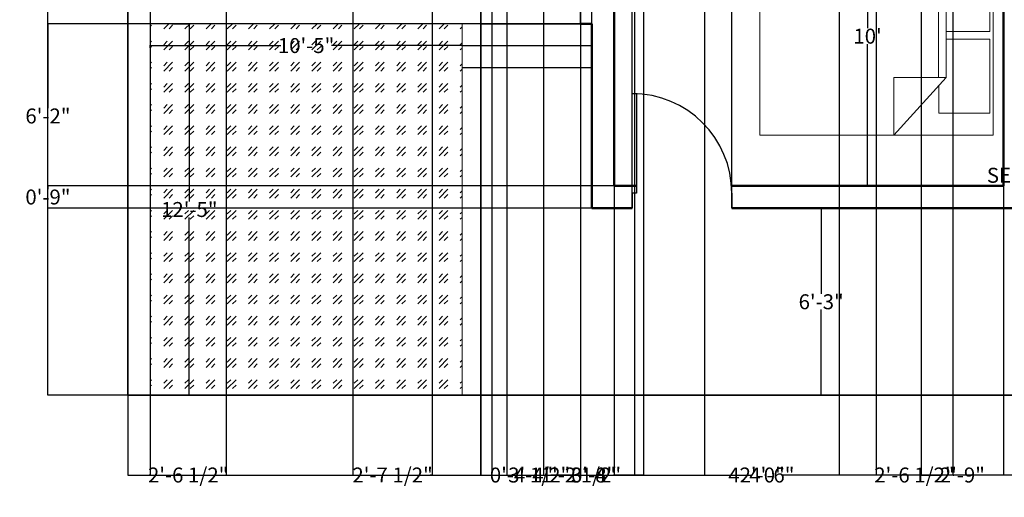
# Model space of a CAD drawing. Units: inches. Extents: x -56 to 545, y -536 to 185.
# Tile 1 of 7: x -49 to 345, y -536 to -344. Entities that reach past the tile are written whole.
import ezdxf

# ---------------------------------------------------------------- set-up
doc = ezdxf.new("R2010")
doc.units = ezdxf.units.IN
doc.header["$MEASUREMENT"] = 0
for name, color, linetype, lineweight in [('A-ANNO-DIMS', 2, 'Continuous', 18), ('A-DOOR', 4, 'Continuous', 25), ('A-FLOR-STRS', 7, 'Continuous', 25), ('A-FURN', 8, 'Continuous', 18), ('A-WALL', 7, 'Continuous', 50), ('C-PROP', 7, 'Continuous', 35), ('L-PLNT-PATT', 3, 'Continuous', 13), ('L-PLNT-TURF', 3, 'Continuous', 18)]:
    doc.layers.add(name, color=color, linetype=linetype, lineweight=lineweight)
doc.styles.get("Standard").update_dxf_attribs({"font": 'arial.ttf'})
doc.dimstyles.get("Standard").update_dxf_attribs({"dimtxt": 6, "dimasz": 0.18, "dimexe": 0.18, "dimexo": 0.0625, "dimgap": 0.09, "dimtad": 0, "dimtih": 1, "dimtoh": 1, "dimdec": 0, "dimzin": 0, "dimdsep": 46, "dimlunit": 3, "dimtxsty": 'Standard', "dimcen": 0.09, "dimclrd": 3, "dimclre": 3, "dimclrt": 3, "dimadec": 0, "dimazin": 0, "dimtfac": 1, "dimtdec": 0, "dimtofl": 0, "dimtmove": 0, "dimatfit": 3, "dimfxl": 1, "dimtolj": 1, "dimtzin": 0, "dimarcsym": 0})

# ---------------------------------------------------------------- blocks, each defined once
blk = doc.blocks.new('CAMAKING')
for points in [[(0.8635, 0), (-0.8635, 0)], [(-0.8635, -2.0147), (-0.8635, 0)], [(0.8635, 0), (0.8635, -2.0147)], [(-0.6723, -0.4077), (-0.6723, -0.0281)], [(-0.6723, -0.0281), (-0.0328, -0.0281)], [(-0.0328, -0.0281), (-0.0328, -0.4077)], [(0.6716, -0.027), (0.0319, -0.027)], [(0.0319, -0.027), (0.0319, -0.4077)], [(0.6716, -0.4686), (0.6716, -0.027)], [(0.3645, -0.4056), (-0.8635, -0.4056)], [(0.8635, -0.857), (0.3645, -0.4056)], [(0.3645, -0.4702), (0.3645, -0.4056)], [(-0.8635, -0.4702), (0.3645, -0.4702)], [(0.3645, -0.4702), (0.3645, -0.857)], [(0.4362, -0.4686), (0.6716, -0.4686)], [(0.3645, -0.857), (0.8635, -0.857)], [(0.8635, -2.0147), (-0.8635, -2.0147)]]:
    blk.add_lwpolyline(points)
blk = doc.blocks.new('*U7')
for p, q in [((0, 0), (0, -6)), ((40, 0), (40, -6))]:
    blk.add_line(p, q)
blk.add_lwpolyline([(0, 0), (0, 40), (1.75, 40), (1.75, 0)], close=True)
blk.add_arc((0, 0), 40, 0, 90)
blk = doc.blocks.new('*D14')
at = {"layer": 'A-ANNO-DIMS', "color": 0, "lineweight": -2, "transparency": 16777216}
for p, q in [((290.53, -291.02), (290.53, -347.69)), ((290.6, -290.84), (290.71, -290.84)), ((290.53, -410.66), (290.53, -353.99)), ((290.6, -410.84), (290.71, -410.84))]:
    blk.add_line(p, q, dxfattribs=at)
at = {"layer": 'A-ANNO-DIMS', "color": 0, "transparency": 16777216}
for points in [[(290.5, -291.02), (290.56, -291.02), (290.53, -290.84)], [(290.5, -410.66), (290.56, -410.66), (290.53, -410.84)]]:
    blk.add_solid(points, dxfattribs=at)
at = {"layer": 'Defpoints', "color": 0, "transparency": 16777216}
for p in [(290.53, -290.84), (290.53, -290.84), (290.53, -410.84)]:
    blk.add_point(p, dxfattribs=at)
at = {"layer": 'A-ANNO-DIMS', "color": 0, "transparency": 16777216, "insert": (290.53, -350.84), "char_height": 6, "attachment_point": 5}
blk.add_mtext("\\A1;10'", dxfattribs=at)
blk = doc.blocks.new('*D15')
at = {"layer": 'A-ANNO-DIMS', "color": 0, "lineweight": -2, "transparency": 16777216}
for p, q in [((11.7, -345.84), (18.9, -345.84)), ((18.72, -346.02), (18.72, -417.19)), ((18.72, -494.66), (18.72, -423.49)), ((11.7, -494.84), (18.9, -494.84))]:
    blk.add_line(p, q, dxfattribs=at)
at = {"layer": 'A-ANNO-DIMS', "color": 0, "transparency": 16777216}
for points in [[(18.69, -346.02), (18.75, -346.02), (18.72, -345.84)], [(18.69, -494.66), (18.75, -494.66), (18.72, -494.84)]]:
    blk.add_solid(points, dxfattribs=at)
at = {"layer": 'Defpoints', "color": 0, "transparency": 16777216}
for p in [(11.63, -345.84), (11.63, -494.84), (18.72, -494.84)]:
    blk.add_point(p, dxfattribs=at)
at = {"layer": 'A-ANNO-DIMS', "color": 0, "transparency": 16777216, "insert": (18.72, -420.34), "char_height": 6, "attachment_point": 5}
blk.add_mtext('\\A1;12\'-5"', dxfattribs=at)
blk = doc.blocks.new('*D16')
at = {"layer": 'A-ANNO-DIMS', "color": 0, "lineweight": -2, "transparency": 16777216}
for p, q in [((3.03, -355.56), (3.03, -354.43)), ((3.21, -354.61), (55.42, -354.61)), ((127.85, -354.61), (75.65, -354.61)), ((128.03, -354.55), (128.03, -354.43))]:
    blk.add_line(p, q, dxfattribs=at)
at = {"layer": 'A-ANNO-DIMS', "color": 0, "transparency": 16777216}
for points in [[(3.21, -354.58), (3.21, -354.64), (3.03, -354.61)], [(127.85, -354.58), (127.85, -354.64), (128.03, -354.61)]]:
    blk.add_solid(points, dxfattribs=at)
at = {"layer": 'Defpoints', "color": 0, "transparency": 16777216}
for p in [(128.03, -354.61), (128.03, -354.61), (3.03, -355.62)]:
    blk.add_point(p, dxfattribs=at)
at = {"layer": 'A-ANNO-DIMS', "color": 0, "transparency": 16777216, "insert": (65.53, -354.61), "char_height": 6, "attachment_point": 5}
blk.add_mtext('\\A1;10\'-5"', dxfattribs=at)
blk = doc.blocks.new('*D34')
at = {"layer": 'A-ANNO-DIMS', "color": 0, "lineweight": -2, "transparency": 16777216}
for p, q in [((263.14, -419.84), (272.12, -419.84)), ((271.94, -420.02), (271.94, -454.19)), ((271.94, -494.66), (271.94, -460.5)), ((263.14, -494.84), (272.12, -494.84))]:
    blk.add_line(p, q, dxfattribs=at)
at = {"layer": 'A-ANNO-DIMS', "color": 0, "transparency": 16777216}
for points in [[(271.91, -420.02), (271.97, -420.02), (271.94, -419.84)], [(271.91, -494.66), (271.97, -494.66), (271.94, -494.84)]]:
    blk.add_solid(points, dxfattribs=at)
at = {"layer": 'Defpoints', "color": 0, "transparency": 16777216}
for p in [(263.08, -419.84), (263.08, -494.84), (271.94, -494.84)]:
    blk.add_point(p, dxfattribs=at)
at = {"layer": 'A-ANNO-DIMS', "color": 0, "transparency": 16777216, "insert": (271.94, -457.34), "char_height": 6, "attachment_point": 5}
blk.add_mtext('\\A1;6\'-3"', dxfattribs=at)
blk = doc.blocks.new('*D49')
at = {"layer": 'A-ANNO-DIMS', "color": 3, "lineweight": -2, "transparency": 16777216}
for p, q in [((389.1, -321.67), (363.5, -321.67)), ((363.68, -321.85), (363.68, -403.43)), ((363.68, -491.39), (363.68, -409.81)), ((389.1, -491.57), (363.5, -491.57))]:
    blk.add_line(p, q, dxfattribs=at)
at = {"layer": 'A-ANNO-DIMS', "color": 3, "transparency": 16777216}
for points in [[(363.65, -321.85), (363.71, -321.85), (363.68, -321.67)], [(363.65, -491.39), (363.71, -491.39), (363.68, -491.57)]]:
    blk.add_solid(points, dxfattribs=at)
at = {"layer": 'Defpoints', "color": 0, "transparency": 16777216}
for p in [(389.16, -321.67), (363.68, -491.57), (389.16, -491.57)]:
    blk.add_point(p, dxfattribs=at)
at = {"layer": 'A-ANNO-DIMS', "color": 3, "transparency": 16777216, "insert": (363.68, -406.62), "char_height": 6, "attachment_point": 5}
blk.add_mtext('\\A1;SEDAN 14\'-2"', dxfattribs=at)
blk = doc.blocks.new('*D51')
at = {"layer": 'A-ANNO-DIMS', "color": 3, "lineweight": -2, "transparency": 16777216}
for p, q in [((498.03, -491.9), (498.03, -526.99)), ((-5.97, -494.9), (-5.97, -526.99)), ((-5.79, -526.81), (235.52, -526.81)), ((497.85, -526.81), (256.55, -526.81))]:
    blk.add_line(p, q, dxfattribs=at)
at = {"layer": 'A-ANNO-DIMS', "color": 3, "transparency": 16777216}
for points in [[(-5.79, -526.78), (-5.79, -526.84), (-5.97, -526.81)], [(497.85, -526.78), (497.85, -526.84), (498.03, -526.81)]]:
    blk.add_solid(points, dxfattribs=at)
at = {"layer": 'Defpoints', "color": 0, "transparency": 16777216}
for p in [(498.03, -491.84), (-5.97, -494.84), (498.03, -526.81)]:
    blk.add_point(p, dxfattribs=at)
at = {"layer": 'A-ANNO-DIMS', "color": 3, "transparency": 16777216, "insert": (246.03, -526.81), "char_height": 6, "attachment_point": 5}
blk.add_mtext('\\A1;42\'-0"', dxfattribs=at)
blk = doc.blocks.new('*D52')
at = {"layer": 'A-ANNO-DIMS', "color": 3, "lineweight": -2, "transparency": 16777216}
for p, q in [((-6.03, 93.16), (-38.11, 93.16)), ((-37.93, 92.98), (-37.93, -197.69)), ((-37.93, -494.66), (-37.93, -203.99)), ((-6.03, -494.84), (-38.11, -494.84))]:
    blk.add_line(p, q, dxfattribs=at)
at = {"layer": 'A-ANNO-DIMS', "color": 3, "transparency": 16777216}
for points in [[(-37.96, 92.98), (-37.9, 92.98), (-37.93, 93.16)], [(-37.96, -494.66), (-37.9, -494.66), (-37.93, -494.84)]]:
    blk.add_solid(points, dxfattribs=at)
at = {"layer": 'Defpoints', "color": 0, "transparency": 16777216}
for p in [(-5.97, 93.16), (-37.93, -494.84), (-5.97, -494.84)]:
    blk.add_point(p, dxfattribs=at)
at = {"layer": 'A-ANNO-DIMS', "color": 3, "transparency": 16777216, "insert": (-37.93, -200.84), "char_height": 6, "attachment_point": 5}
blk.add_mtext('\\A1;49\'-0"', dxfattribs=at)
blk = doc.blocks.new('*D53')
at = {"layer": 'A-ANNO-DIMS', "color": 3, "lineweight": -2, "transparency": 16777216}
for p, q in [((179.97, -345.84), (-38.11, -345.84)), ((-37.93, -346.02), (-37.93, -379.69)), ((-37.93, -419.66), (-37.93, -385.99)), ((179.97, -419.84), (-38.11, -419.84))]:
    blk.add_line(p, q, dxfattribs=at)
at = {"layer": 'A-ANNO-DIMS', "color": 3, "transparency": 16777216}
for points in [[(-37.96, -346.02), (-37.9, -346.02), (-37.93, -345.84)], [(-37.96, -419.66), (-37.9, -419.66), (-37.93, -419.84)]]:
    blk.add_solid(points, dxfattribs=at)
at = {"layer": 'Defpoints', "color": 0, "transparency": 16777216}
for p in [(180.03, -345.84), (-37.93, -419.84), (180.03, -419.84)]:
    blk.add_point(p, dxfattribs=at)
at = {"layer": 'A-ANNO-DIMS', "color": 3, "transparency": 16777216, "insert": (-37.93, -382.84), "char_height": 6, "attachment_point": 5}
blk.add_mtext('\\A1;6\'-2"', dxfattribs=at)
blk = doc.blocks.new('*D54')
at = {"layer": 'A-ANNO-DIMS', "color": 3, "lineweight": -2, "transparency": 16777216}
for p, q in [((188.97, -410.84), (-38.11, -410.84)), ((-37.93, -411.02), (-37.93, -412.19)), ((179.97, -419.84), (-38.11, -419.84)), ((-37.93, -419.66), (-37.93, -418.49))]:
    blk.add_line(p, q, dxfattribs=at)
at = {"layer": 'A-ANNO-DIMS', "color": 3, "transparency": 16777216}
for points in [[(-37.96, -411.02), (-37.9, -411.02), (-37.93, -410.84)], [(-37.96, -419.66), (-37.9, -419.66), (-37.93, -419.84)]]:
    blk.add_solid(points, dxfattribs=at)
at = {"layer": 'Defpoints', "color": 0, "transparency": 16777216}
for p in [(189.03, -410.84), (-37.93, -419.84), (180.03, -419.84)]:
    blk.add_point(p, dxfattribs=at)
at = {"layer": 'A-ANNO-DIMS', "color": 3, "transparency": 16777216, "insert": (-37.93, -415.34), "char_height": 6, "attachment_point": 5}
blk.add_mtext('\\A1;0\'-9"', dxfattribs=at)
blk = doc.blocks.new('*D60')
at = {"layer": 'A-ANNO-DIMS', "color": 3, "lineweight": -2, "transparency": 16777216}
for p, q in [((135.54, -345.9), (135.54, -526.99)), ((175.54, -345.9), (175.54, -526.99)), ((135.72, -526.81), (147.48, -526.81)), ((175.36, -526.81), (163.61, -526.81))]:
    blk.add_line(p, q, dxfattribs=at)
at = {"layer": 'A-ANNO-DIMS', "color": 3, "transparency": 16777216}
for points in [[(135.72, -526.78), (135.72, -526.84), (135.54, -526.81)], [(175.36, -526.78), (175.36, -526.84), (175.54, -526.81)]]:
    blk.add_solid(points, dxfattribs=at)
at = {"layer": 'Defpoints', "color": 0, "transparency": 16777216}
for p in [(135.54, -345.84), (175.54, -345.84), (175.54, -526.81)]:
    blk.add_point(p, dxfattribs=at)
at = {"layer": 'A-ANNO-DIMS', "color": 3, "transparency": 16777216, "insert": (155.54, -526.81), "char_height": 6, "attachment_point": 5}
blk.add_mtext('\\A1;3\'-4"', dxfattribs=at)
blk = doc.blocks.new('*D61')
at = {"layer": 'A-ANNO-DIMS', "color": 3, "lineweight": -2, "transparency": 16777216}
for p, q in [((175.54, -345.78), (175.54, 176.3)), ((175.72, 176.12), (179.85, 176.12)), ((180.03, -345.78), (180.03, 176.3)), ((180.03, 176.12), (180.21, 176.12))]:
    blk.add_line(p, q, dxfattribs=at)
at = {"layer": 'A-ANNO-DIMS', "color": 3, "transparency": 16777216}
for points in [[(175.72, 176.15), (175.72, 176.09), (175.54, 176.12)], [(179.85, 176.15), (179.85, 176.09), (180.03, 176.12)]]:
    blk.add_solid(points, dxfattribs=at)
at = {"layer": 'Defpoints', "color": 0, "transparency": 16777216}
for p in [(180.03, 176.12), (175.54, -345.84), (180.03, -345.84)]:
    blk.add_point(p, dxfattribs=at)
at = {"layer": 'A-ANNO-DIMS', "color": 3, "transparency": 16777216, "insert": (195.27, 176.12), "char_height": 6, "attachment_point": 5}
blk.add_mtext('\\A1;0\'-4 1/2"', dxfattribs=at)
blk = doc.blocks.new('*D62')
at = {"layer": 'A-ANNO-DIMS', "color": 3, "lineweight": -2, "transparency": 16777216}
for p, q in [((196.14, -419.78), (196.14, 176.3)), ((196.32, 176.12), (208.08, 176.12)), ((235.96, 176.12), (224.21, 176.12)), ((236.14, -419.78), (236.14, 176.3))]:
    blk.add_line(p, q, dxfattribs=at)
at = {"layer": 'A-ANNO-DIMS', "color": 3, "transparency": 16777216}
for points in [[(196.32, 176.15), (196.32, 176.09), (196.14, 176.12)], [(235.96, 176.15), (235.96, 176.09), (236.14, 176.12)]]:
    blk.add_solid(points, dxfattribs=at)
at = {"layer": 'Defpoints', "color": 0, "transparency": 16777216}
for p in [(236.14, 176.12), (196.14, -419.84), (236.14, -419.84)]:
    blk.add_point(p, dxfattribs=at)
at = {"layer": 'A-ANNO-DIMS', "color": 3, "transparency": 16777216, "insert": (216.14, 176.12), "char_height": 6, "attachment_point": 5}
blk.add_mtext('\\A1;3\'-4"', dxfattribs=at)
blk = doc.blocks.new('*D63')
at = {"layer": 'A-ANNO-DIMS', "color": 3, "lineweight": -2, "transparency": 16777216}
for p, q in [((189.03, -410.78), (189.03, 176.3)), ((189.21, 176.12), (195.96, 176.12)), ((196.14, -419.78), (196.14, 176.3)), ((196.14, 176.12), (196.32, 176.12))]:
    blk.add_line(p, q, dxfattribs=at)
at = {"layer": 'A-ANNO-DIMS', "color": 3, "transparency": 16777216}
for points in [[(189.21, 176.15), (189.21, 176.09), (189.03, 176.12)], [(195.96, 176.15), (195.96, 176.09), (196.14, 176.12)]]:
    blk.add_solid(points, dxfattribs=at)
at = {"layer": 'Defpoints', "color": 0, "transparency": 16777216}
for p in [(196.14, 176.12), (189.03, -410.84), (196.14, -419.84)]:
    blk.add_point(p, dxfattribs=at)
at = {"layer": 'A-ANNO-DIMS', "color": 3, "transparency": 16777216, "insert": (204.39, 176.12), "char_height": 6, "attachment_point": 5}
blk.add_mtext('\\A1;0\'-7"', dxfattribs=at)
blk = doc.blocks.new('*D64')
at = {"layer": 'A-ANNO-DIMS', "color": 3, "lineweight": -2, "transparency": 16777216}
for p, q in [((293.965457, -119.903074), (293.965457, -526.985574)), ((324.688571, -119.903074), (324.688571, -526.985574)), ((293.785457, -526.805574), (293.605457, -526.805574)), ((324.868571, -526.805574), (325.048571, -526.805574))]:
    blk.add_line(p, q, dxfattribs=at)
at = {"layer": 'A-ANNO-DIMS', "color": 3, "transparency": 16777216}
for points in [[(293.785457, -526.775574), (293.785457, -526.835574), (293.965457, -526.805574)], [(324.868571, -526.775574), (324.868571, -526.835574), (324.688571, -526.805574)]]:
    blk.add_solid(points, dxfattribs=at)
at = {"layer": 'Defpoints', "color": 0, "transparency": 16777216}
for p in [(293.965457, -119.840574), (324.688571, -119.840574), (324.688571, -526.805574)]:
    blk.add_point(p, dxfattribs=at)
at = {"layer": 'A-ANNO-DIMS', "color": 3, "transparency": 16777216, "insert": (309.327014, -526.805574), "char_height": 6, "attachment_point": 5}
blk.add_mtext('\\A1;2\'-6 1/2"', dxfattribs=at)
blk = doc.blocks.new('*D65')
at = {"layer": 'A-ANNO-DIMS', "color": 3, "lineweight": -2, "transparency": 16777216}
for p, q in [((160.69, -65.9), (160.69, -526.99)), ((200.69, -65.9), (200.69, -526.99)), ((160.87, -526.81), (172.63, -526.81)), ((200.51, -526.81), (188.76, -526.81))]:
    blk.add_line(p, q, dxfattribs=at)
at = {"layer": 'A-ANNO-DIMS', "color": 3, "transparency": 16777216}
for points in [[(160.87, -526.78), (160.87, -526.84), (160.69, -526.81)], [(200.51, -526.78), (200.51, -526.84), (200.69, -526.81)]]:
    blk.add_solid(points, dxfattribs=at)
at = {"layer": 'Defpoints', "color": 0, "transparency": 16777216}
for p in [(160.69, -65.84), (200.69, -65.84), (200.69, -526.81)]:
    blk.add_point(p, dxfattribs=at)
at = {"layer": 'A-ANNO-DIMS', "color": 3, "transparency": 16777216, "insert": (180.69, -526.81), "char_height": 6, "attachment_point": 5}
blk.add_mtext('\\A1;3\'-4"', dxfattribs=at)
blk = doc.blocks.new('*D66')
at = {"layer": 'A-ANNO-DIMS', "color": 3, "lineweight": -2, "transparency": 16777216}
for p, q in [((146.03, -65.9), (146.03, -526.99)), ((160.69, -65.9), (160.69, -526.99)), ((146.21, -526.81), (160.51, -526.81)), ((160.69, -526.81), (160.87, -526.81))]:
    blk.add_line(p, q, dxfattribs=at)
at = {"layer": 'A-ANNO-DIMS', "color": 3, "transparency": 16777216}
for points in [[(146.21, -526.78), (146.21, -526.84), (146.03, -526.81)], [(160.51, -526.78), (160.51, -526.84), (160.69, -526.81)]]:
    blk.add_solid(points, dxfattribs=at)
at = {"layer": 'Defpoints', "color": 0, "transparency": 16777216}
for p in [(146.03, -65.84), (160.69, -65.84), (160.69, -526.81)]:
    blk.add_point(p, dxfattribs=at)
at = {"layer": 'A-ANNO-DIMS', "color": 3, "transparency": 16777216, "insert": (175.65, -526.81), "char_height": 6, "attachment_point": 5}
blk.add_mtext('\\A1;1\'-2 1/2"', dxfattribs=at)
blk = doc.blocks.new('*D69')
at = {"layer": 'A-ANNO-DIMS', "color": 3, "lineweight": -2, "transparency": 16777216}
for p, q in [((189.03, -290.9), (189.03, -526.99)), ((197.13, -290.9), (197.13, -526.99)), ((189.03, -526.81), (188.85, -526.81)), ((196.95, -526.81), (189.21, -526.81))]:
    blk.add_line(p, q, dxfattribs=at)
at = {"layer": 'A-ANNO-DIMS', "color": 3, "transparency": 16777216}
for points in [[(189.21, -526.78), (189.21, -526.84), (189.03, -526.81)], [(196.95, -526.78), (196.95, -526.84), (197.13, -526.81)]]:
    blk.add_solid(points, dxfattribs=at)
at = {"layer": 'Defpoints', "color": 0, "transparency": 16777216}
for p in [(189.03, -290.84), (197.13, -290.84), (189.03, -526.81)]:
    blk.add_point(p, dxfattribs=at)
at = {"layer": 'A-ANNO-DIMS', "color": 3, "transparency": 16777216, "insert": (180.79, -526.81), "char_height": 6, "attachment_point": 5}
blk.add_mtext('\\A1;0\'-8"', dxfattribs=at)
blk = doc.blocks.new('*D73')
at = {"layer": 'A-ANNO-DIMS', "color": 3, "lineweight": -2, "transparency": 16777216}
for p, q in [((135.38, 28.1), (135.38, -526.99)), ((140.03, 28.1), (140.03, -526.99)), ((135.56, -526.81), (139.85, -526.81)), ((140.03, -526.81), (140.21, -526.81))]:
    blk.add_line(p, q, dxfattribs=at)
at = {"layer": 'A-ANNO-DIMS', "color": 3, "transparency": 16777216}
for points in [[(135.56, -526.78), (135.56, -526.84), (135.38, -526.81)], [(139.85, -526.78), (139.85, -526.84), (140.03, -526.81)]]:
    blk.add_solid(points, dxfattribs=at)
at = {"layer": 'Defpoints', "color": 0, "transparency": 16777216}
for p in [(135.38, 28.16), (140.03, 28.16), (140.03, -526.81)]:
    blk.add_point(p, dxfattribs=at)
at = {"layer": 'A-ANNO-DIMS', "color": 3, "transparency": 16777216, "insert": (155.27, -526.81), "char_height": 6, "attachment_point": 5}
blk.add_mtext('\\A1;0\'-4 1/2"', dxfattribs=at)
blk = doc.blocks.new('*D75')
at = {"layer": 'A-ANNO-DIMS', "color": 3, "lineweight": -2, "transparency": 16777216}
for p, q in [((33.5, -201.14), (33.5, -526.99)), ((3.03, -229.9), (3.03, -526.99)), ((2.85, -526.81), (2.67, -526.81)), ((33.68, -526.81), (33.86, -526.81))]:
    blk.add_line(p, q, dxfattribs=at)
at = {"layer": 'A-ANNO-DIMS', "color": 3, "transparency": 16777216}
for points in [[(2.85, -526.78), (2.85, -526.84), (3.03, -526.81)], [(33.68, -526.78), (33.68, -526.84), (33.5, -526.81)]]:
    blk.add_solid(points, dxfattribs=at)
at = {"layer": 'Defpoints', "color": 0, "transparency": 16777216}
for p in [(33.5, -201.08), (3.03, -229.84), (33.5, -526.81)]:
    blk.add_point(p, dxfattribs=at)
at = {"layer": 'A-ANNO-DIMS', "color": 3, "transparency": 16777216, "insert": (18.27, -526.81), "char_height": 6, "attachment_point": 5}
blk.add_mtext('\\A1;2\'-6 1/2"', dxfattribs=at)
blk = doc.blocks.new('*D81')
at = {"layer": 'A-ANNO-DIMS', "color": 3, "lineweight": -2, "transparency": 16777216}
for p, q in [((345.03, 60.47), (345.03, -526.99)), ((312.03, 49.97), (312.03, -526.99)), ((312.21, -526.81), (320.42, -526.81)), ((344.85, -526.81), (336.65, -526.81))]:
    blk.add_line(p, q, dxfattribs=at)
at = {"layer": 'A-ANNO-DIMS', "color": 3, "transparency": 16777216}
for points in [[(312.21, -526.78), (312.21, -526.84), (312.03, -526.81)], [(344.85, -526.78), (344.85, -526.84), (345.03, -526.81)]]:
    blk.add_solid(points, dxfattribs=at)
at = {"layer": 'Defpoints', "color": 0, "transparency": 16777216}
for p in [(345.03, 60.53), (312.03, 50.03), (312.03, -526.81)]:
    blk.add_point(p, dxfattribs=at)
at = {"layer": 'A-ANNO-DIMS', "color": 3, "transparency": 16777216, "insert": (328.53, -526.81), "char_height": 6, "attachment_point": 5}
blk.add_mtext('\\A1;2\'-9"', dxfattribs=at)
blk = doc.blocks.new('*D83')
at = {"layer": 'A-ANNO-DIMS', "color": 3, "lineweight": -2, "transparency": 16777216}
for p, q in [((225.22, -238.28), (225.22, -526.99)), ((279.14, -238.28), (279.14, -526.99)), ((225.4, -526.81), (243.99, -526.81)), ((278.96, -526.81), (260.36, -526.81))]:
    blk.add_line(p, q, dxfattribs=at)
at = {"layer": 'A-ANNO-DIMS', "color": 3, "transparency": 16777216}
for points in [[(225.4, -526.78), (225.4, -526.84), (225.22, -526.81)], [(278.96, -526.78), (278.96, -526.84), (279.14, -526.81)]]:
    blk.add_solid(points, dxfattribs=at)
at = {"layer": 'Defpoints', "color": 0, "transparency": 16777216}
for p in [(225.22, -238.22), (279.14, -238.22), (279.14, -526.81)]:
    blk.add_point(p, dxfattribs=at)
at = {"layer": 'A-ANNO-DIMS', "color": 3, "transparency": 16777216, "insert": (252.18, -526.81), "char_height": 6, "attachment_point": 5}
blk.add_mtext('\\A1;4\'-6"', dxfattribs=at)
blk = doc.blocks.new('*D85')
at = {"layer": 'A-ANNO-DIMS', "color": 3, "lineweight": -2, "transparency": 16777216}
for p, q in [((84.32, -227.78), (84.32, -526.99)), ((116.03, -229.9), (116.03, -526.99)), ((84.5, -526.81), (85.07, -526.81)), ((115.85, -526.81), (115.28, -526.81))]:
    blk.add_line(p, q, dxfattribs=at)
at = {"layer": 'A-ANNO-DIMS', "color": 3, "transparency": 16777216}
for points in [[(84.5, -526.78), (84.5, -526.84), (84.32, -526.81)], [(115.85, -526.78), (115.85, -526.84), (116.03, -526.81)]]:
    blk.add_solid(points, dxfattribs=at)
at = {"layer": 'Defpoints', "color": 0, "transparency": 16777216}
for p in [(84.32, -227.71), (116.03, -229.84), (116.03, -526.81)]:
    blk.add_point(p, dxfattribs=at)
at = {"layer": 'A-ANNO-DIMS', "color": 3, "transparency": 16777216, "insert": (100.18, -526.81), "char_height": 6, "attachment_point": 5}
blk.add_mtext('\\A1;2\'-7 1/2"', dxfattribs=at)

msp = doc.modelspace()

# ---------------------------------------------------------------- hatches: boundary and pattern name
at = {"layer": 'L-PLNT-PATT'}
h = msp.add_hatch(dxfattribs=at)
h.set_pattern_fill('GOST_GLASS', color=256)
h.set_pattern_definition([(45, (0, 0), (8.48528, 0), [5, -7]), (45, (2.1213, 0), (8.48528, 0), [2, -10]), (45, (0, 2.1213), (8.48528, 0), [2, -10])])
h.paths.add_polyline_path([(128.03, -345.84), (3.03, -345.84), (3.03, -494.84), (122.03, -494.84), (128.03, -494.84)])

# ---------------------------------------------------------------- linework, layer by layer
at = {"layer": 'A-FLOR-STRS'}
for p, q in [((135.54, -345.84), (175.54, -345.84)), ((128.03, -354.61), (180.03, -354.61)), ((128.03, -363.36), (180.03, -363.36))]:
    msp.add_line(p, q, dxfattribs=at)
at = {"layer": 'A-WALL'}
for p, q in [((189.03, -290.84), (189.03, -345.84)), ((345.03, -290.84), (345.03, -410.84)), ((175.54, -345.84), (180.03, -345.84)), ((180.03, -345.84), (180.03, -419.84)), ((189.03, -345.84), (189.03, -410.84)), ((189.03, -410.84), (197.89, -410.84)), ((236.03, -410.84), (345.03, -410.84)), ((180.03, -419.84), (196.14, -419.84)), ((236.14, -419.84), (354.03, -419.84))]:
    msp.add_line(p, q, dxfattribs=at)
at = {"layer": 'C-PROP'}
for p, q in [((-5.97, 93.16), (-5.97, -494.84)), ((-5.97, -494.84), (122.03, -494.84)), ((122.03, -494.84), (495.03, -494.84))]:
    msp.add_line(p, q, dxfattribs=at)
at = {"layer": 'L-PLNT-TURF'}
for p, q in [((3.03, -345.84), (3.03, -494.84)), ((3.03, -345.84), (135.54, -345.84)), ((128.03, -345.84), (128.03, -494.84))]:
    msp.add_line(p, q, dxfattribs=at)

# ---------------------------------------------------------------- block references
at = {"layer": 'A-DOOR'}
for p in [(135.54, -339.84), (196.14, -413.84)]:
    msp.add_blockref('*U7', p, dxfattribs=at)
at = {"layer": 'A-FURN', "xscale": 46.34928316146463, "yscale": 46.34928316146463, "zscale": 46.34928316146463, "rotation": 270}
msp.add_blockref('CAMAKING', (340.81, -350.54), dxfattribs=at)

# ---------------------------------------------------------------- dimensions: what is measured, and where the dimension line sits
at = {"layer": 'A-ANNO-DIMS'}
for base, p1, p2, override, picture, middle in [((180.03, 176.12), (175.54, -345.84), (180.03, -345.84), {"dimdec": 1, "dimlfac": 1, "dimrnd": 0, "dimzin": 1, "dimdsep": 46, "dimlunit": 4, "dimfrac": 2}, '*D61', (195.27, 176.12)), ((196.14, 176.12), (189.03, -410.84), (196.14, -419.84), {"dimdec": 1, "dimlfac": 1, "dimrnd": 0, "dimzin": 1, "dimdsep": 46, "dimlunit": 4, "dimfrac": 2}, '*D63', (204.39, 176.12)), ((236.14, 176.12), (196.14, -419.84), (236.14, -419.84), {"dimdec": 1, "dimlfac": 1, "dimrnd": 0, "dimzin": 1, "dimdsep": 46, "dimlunit": 4, "dimfrac": 2}, '*D62', (216.14, 176.12)), ((312.03, -526.81), (345.03, 60.53), (312.03, 50.03), {"dimdec": 1, "dimlfac": 1, "dimrnd": 0, "dimzin": 1, "dimdsep": 46, "dimlunit": 4, "dimfrac": 2}, '*D81', (328.53, -526.81)), ((140.0343, -526.8056), (135.3838, 28.1594), (140.0343, 28.1594), {"dimdec": 1, "dimlfac": 1, "dimrnd": 0, "dimzin": 1, "dimdsep": 46, "dimlunit": 4, "dimfrac": 2}, '*D73', (155.2695, -526.8056)), ((160.69, -526.81), (146.03, -65.84), (160.69, -65.84), {"dimdec": 1, "dimlfac": 1, "dimrnd": 0, "dimzin": 1, "dimdsep": 46, "dimlunit": 4, "dimfrac": 2}, '*D66', (175.65, -526.81)), ((200.69, -526.81), (160.69, -65.84), (200.69, -65.84), {"dimdec": 1, "dimlfac": 1, "dimrnd": 0, "dimzin": 1, "dimdsep": 46, "dimlunit": 4, "dimfrac": 2}, '*D65', (180.69, -526.81)), ((324.69, -526.81), (293.97, -119.84), (324.69, -119.84), {"dimdec": 1, "dimlfac": 1, "dimrnd": 0, "dimzin": 1, "dimdsep": 46, "dimlunit": 4, "dimfrac": 2}, '*D64', (309.33, -526.81)), ((33.5, -526.81), (3.03, -229.84), (33.5, -201.08), {"dimdec": 1, "dimlfac": 1, "dimrnd": 0, "dimzin": 1, "dimdsep": 46, "dimlunit": 4, "dimfrac": 2}, '*D75', (18.27, -526.81)), ((116.03, -526.81), (84.32, -227.71), (116.03, -229.84), {"dimdec": 1, "dimlfac": 1, "dimrnd": 0, "dimzin": 1, "dimdsep": 46, "dimlunit": 4, "dimfrac": 2}, '*D85', (100.18, -526.81)), ((279.14, -526.81), (225.22, -238.22), (279.14, -238.22), {"dimdec": 1, "dimlfac": 1, "dimrnd": 0, "dimzin": 1, "dimdsep": 46, "dimlunit": 4, "dimfrac": 2}, '*D83', (252.18, -526.81)), ((189.03, -526.81), (197.13, -290.84), (189.03, -290.84), {"dimdec": 1, "dimlfac": 1, "dimrnd": 0, "dimzin": 1, "dimdsep": 46, "dimlunit": 4, "dimfrac": 2}, '*D69', (180.79, -526.81)), ((175.54, -526.81), (135.54, -345.84), (175.54, -345.84), {"dimdec": 1, "dimlfac": 1, "dimrnd": 0, "dimzin": 1, "dimdsep": 46, "dimlunit": 4, "dimfrac": 2}, '*D60', (155.54, -526.81)), ((128.03, -354.61), (3.03, -355.62), (128.03, -354.61), {"dimclrd": 0, "dimclre": 0, "dimclrt": 0}, '*D16', (65.53, -354.61)), ((498.03, -526.81), (-5.97, -494.84), (498.03, -491.84), {"dimdec": 1, "dimlfac": 1, "dimrnd": 0, "dimzin": 1, "dimdsep": 46, "dimlunit": 4, "dimfrac": 2}, '*D51', (246.03, -526.81))]:
    dim = msp.add_linear_dim(base=base, p1=p1, p2=p2, dimstyle='Standard', override=override, dxfattribs=at)
    dim.commit()
    dim.dimension.update_dxf_attribs({"geometry": picture, "text_midpoint": middle})
for base, p1, p2, override, picture, middle in [((-37.93, -494.84), (-5.97, 93.16), (-5.97, -494.84), {"dimdec": 1, "dimlfac": 1, "dimrnd": 0, "dimzin": 1, "dimdsep": 46, "dimlunit": 4, "dimfrac": 2}, '*D52', (-37.93, -200.84)), ((290.53, -290.84), (290.53, -410.84), (290.53, -290.84), {"dimclrd": 0, "dimclre": 0, "dimclrt": 0}, '*D14', (290.53, -350.84)), ((-37.93, -419.84), (180.03, -345.84), (180.03, -419.84), {"dimdec": 1, "dimlfac": 1, "dimrnd": 0, "dimzin": 1, "dimdsep": 46, "dimlunit": 4, "dimfrac": 2}, '*D53', (-37.93, -382.84)), ((18.72, -494.84), (11.63, -345.84), (11.63, -494.84), {"dimclrd": 0, "dimclre": 0, "dimclrt": 0}, '*D15', (18.72, -420.34)), ((-37.93, -419.84), (189.03, -410.84), (180.03, -419.84), {"dimdec": 1, "dimlfac": 1, "dimrnd": 0, "dimzin": 1, "dimdsep": 46, "dimlunit": 4, "dimfrac": 2}, '*D54', (-37.93, -415.34)), ((271.94, -494.84), (263.08, -419.84), (263.08, -494.84), {"dimclrd": 0, "dimclre": 0, "dimclrt": 0}, '*D34', (271.94, -457.34))]:
    dim = msp.add_linear_dim(base=base, p1=p1, p2=p2, angle=90, dimstyle='Standard', override=override, dxfattribs=at)
    dim.commit()
    dim.dimension.update_dxf_attribs({"geometry": picture, "text_midpoint": middle})
dim = msp.add_linear_dim(base=(363.68, -491.57), p1=(389.16, -321.67), p2=(389.16, -491.57), angle=270, text='SEDAN <>', dimstyle='Standard', override={"dimdec": 1, "dimlfac": 1, "dimrnd": 0, "dimzin": 1, "dimdsep": 46, "dimlunit": 4, "dimfrac": 2}, dxfattribs=at)
dim.commit()
dim.dimension.update_dxf_attribs({"geometry": '*D49', "text_midpoint": (363.68, -406.62)})

doc.saveas('drawing.dxf')
